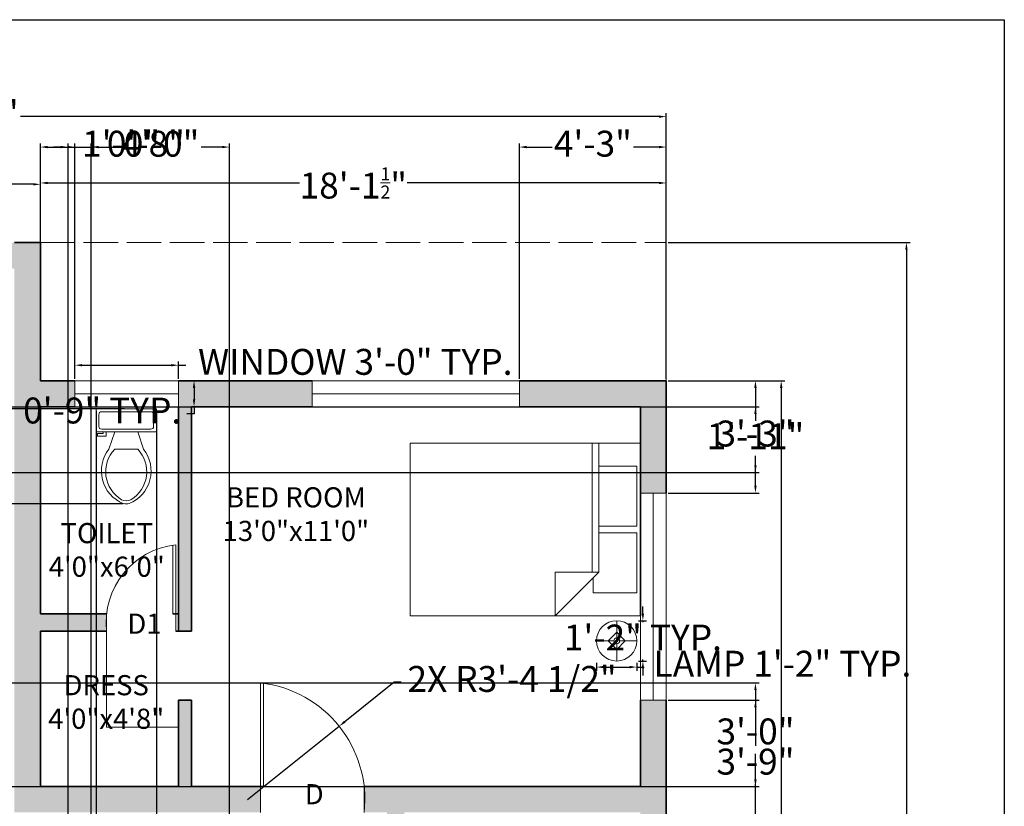
# Model space of a CAD drawing. Units: inches. Extents: x 1942 to 2601, y 2026 to 2623.
# Tile 5 of 5: x 2259 to 2601, y 2350 to 2623. Entities that reach past the tile are written whole.
import ezdxf

# ---------------------------------------------------------------- set-up
doc = ezdxf.new("R2010")
doc.units = ezdxf.units.IN
doc.linetypes.add('ACAD_ISO02W100', pattern=[15, 12, -3])
for name, color, linetype, lineweight in [('A-ANNO-DIMS', 2, 'Continuous', 18), ('A-ANNO-TEXT', 7, 'Continuous', 18), ('A-ANNO-TTLB', 7, 'Continuous', 25), ('A-AREA-IDEN', 7, 'Continuous', 25), ('A-DOOR', 4, 'Continuous', 18), ('A-FLOR-CASE', 8, 'Continuous', 18), ('A-FLOR-FIXT', 8, 'Continuous', 18), ('A-FLOR-OTLN', 8, 'ACAD_ISO02W100', 13), ('A-FURN', 8, 'Continuous', 18), ('A-GLAZ', 2, 'Continuous', 18), ('A-WALL', 7, 'Continuous', 35), ('A-WALL-PATT', 7, 'Continuous', 13)]:
    doc.layers.add(name, color=color, linetype=linetype, lineweight=lineweight)
doc.styles.get("Standard").update_dxf_attribs({"font": 'arial.ttf'})
doc.dimstyles.new('ISO-25', dxfattribs={"dimtxt": 9, "dimasz": 2.5, "dimexe": 1.25, "dimexo": 0.625, "dimgap": 2, "dimtad": 0, "dimtih": 1, "dimtoh": 1, "dimdec": 1, "dimlunit": 4, "dimtxsty": 'Standard', "dimcen": 2.5, "dimadec": 0, "dimazin": 0, "dimtfac": 0.5, "dimtdec": 1, "dimtmove": 0, "dimatfit": 3, "dimfxl": 1, "dimarcsym": 0})

# ---------------------------------------------------------------- blocks, each defined once
blk = doc.blocks.new('Bed - Queen')
for p, q in [((0, -80.00003), (0, 0)), ((0, 0), (59.99999, 0)), ((59.99999, 0), (59.99999, -80.00003)), ((7.99999, -1.2), (28.79998, -1.2)), ((7.99999, -14.4), (7.99999, -1.2)), ((28.79998, -1.2), (28.79998, -14.4)), ((31.19999, -1.2), (51.99999, -1.2)), ((31.19999, -14.4), (31.19999, -1.2)), ((51.99999, -1.2), (51.99999, -16.4)), ((0, -14.4), (44.8, -14.4)), ((44.8, -16.8), (0, -16.8)), ((59.99999, -29.6), (44.8, -14.4)), ((44.8, -14.4), (44.8, -29.6)), ((51.99999, -16.4), (46.79936, -16.4)), ((44.8, -29.6), (59.99999, -29.6)), ((59.99999, -80.00003), (0, -80.00003))]:
    blk.add_line(p, q)
blk = doc.blocks.new('Lamp - Table')
for p, q in [((0, 7), (0, 1)), ((-1, 0), (-7, 0)), ((0, 3), (-3, 0)), ((-3, 0), (0, -3)), ((3, 0), (0, 3)), ((0, -3), (3, 0)), ((1, 0), (7, 0)), ((0, -1), (0, -7))]:
    blk.add_line(p, q)
for radius in [7, 1]:
    blk.add_circle((0, 0), radius)
blk = doc.blocks.new('*U10')
for p, q in [((9.5, -6), (9.5, -2)), ((-10, -8.5), (-8, -8.5)), ((-10, -9.5), (-10, -8.5)), ((-7, -9.5), (-10, -9.5)), ((-8, -8.5), (-8, -8)), ((-7, -8), (-7, -9.5)), ((-4, -8), (-6, -14)), ((4, -8), (6, -14)), ((4, -14), (-4, -14))]:
    blk.add_line(p, q)
blk.add_lwpolyline([(10.5, -8), (10.5, 0), (-10.5, 0), (-10.5, -8)], close=True)
for points in [[(-9.5, -2), (-9.5, -6)], [(8.5, -1), (-8.5, -1)], [(-8.5, -7), (8.5, -7)]]:
    blk.add_lwpolyline(points)
for centre, radius, start, end in [((-8.62, -1.88), 0.884, 81.8699, 188.1301), ((8.62, -1.88), 0.884, 351.8699, 98.1301), ((-8.62, -6.12), 0.884, 171.8699, 278.1301), ((8.62, -6.12), 0.884, 261.8699, 8.1301), ((3.52, -21.58), 12.17, 141.4691, 247.9714), ((4.2, -21.82), 11.33, 136.3677, 238.9468), ((-3.52, -21.58), 12.17, 292.0284, 38.5307), ((-4.2, -21.82), 11.33, 301.053, 43.6321), ((0, -27.88), 4, 245.7318, 294.2682), ((0, -29), 4, 254.8605, 285.1395)]:
    blk.add_arc(centre, radius, start, end)
blk = doc.blocks.new('*D11')
at = {"layer": 'A-ANNO-DIMS', "color": 0, "lineweight": -2, "transparency": 16777216}
for p, q in [((2164.82, 2546.54), (2164.82, 2567.42)), ((2266.32, 2546.54), (2266.32, 2567.42)), ((2167.32, 2566.17), (2199.96, 2566.17)), ((2263.82, 2566.17), (2231.18, 2566.17))]:
    blk.add_line(p, q, dxfattribs=at)
at = {"layer": 'A-ANNO-DIMS', "color": 0, "transparency": 16777216}
for points in [[(2167.32, 2566.58), (2167.32, 2565.75), (2164.82, 2566.17)], [(2263.82, 2566.58), (2263.82, 2565.75), (2266.32, 2566.17)]]:
    blk.add_solid(points, dxfattribs=at)
at = {"layer": 'Defpoints', "color": 0, "transparency": 16777216}
for p in [(2266.32, 2566.17), (2164.82, 2545.91), (2266.32, 2545.91)]:
    blk.add_point(p, dxfattribs=at)
at = {"layer": 'A-ANNO-DIMS', "color": 0, "transparency": 16777216, "insert": (2215.57, 2566.17), "char_height": 9, "attachment_point": 5}
blk.add_mtext('8\'-5{\\H0.5x;\\S1/2;}"', dxfattribs=at)
blk = doc.blocks.new('*D13')
at = {"layer": 'A-ANNO-DIMS', "color": 0, "lineweight": -2, "transparency": 16777216}
for p, q in [((2266.32, 2498.54), (2266.32, 2567.89)), ((2268.82, 2566.64), (2356.39, 2566.64)), ((2481.32, 2566.64), (2393.75, 2566.64)), ((2483.82, 2498.54), (2483.82, 2567.89))]:
    blk.add_line(p, q, dxfattribs=at)
at = {"layer": 'A-ANNO-DIMS', "color": 0, "transparency": 16777216}
for points in [[(2268.82, 2567.06), (2268.82, 2566.23), (2266.32, 2566.64)], [(2481.32, 2567.06), (2481.32, 2566.23), (2483.82, 2566.64)]]:
    blk.add_solid(points, dxfattribs=at)
at = {"layer": 'Defpoints', "color": 0, "transparency": 16777216}
for p in [(2483.82, 2566.64), (2266.32, 2497.91), (2483.82, 2497.91)]:
    blk.add_point(p, dxfattribs=at)
at = {"layer": 'A-ANNO-DIMS', "color": 0, "transparency": 16777216, "insert": (2375.07, 2566.64), "char_height": 9, "attachment_point": 5}
blk.add_mtext('18\'-1{\\H0.5x;\\S1/2;}"', dxfattribs=at)
blk = doc.blocks.new('*D14')
at = {"layer": 'A-ANNO-DIMS', "color": 0, "lineweight": -2, "transparency": 16777216}
for p, q in [((1999.82, 2498.54), (1999.82, 2590.94)), ((2483.82, 2498.54), (2483.82, 2590.94)), ((2002.32, 2589.69), (2224.18, 2589.69)), ((2481.32, 2589.69), (2259.46, 2589.69))]:
    blk.add_line(p, q, dxfattribs=at)
at = {"layer": 'A-ANNO-DIMS', "color": 0, "transparency": 16777216}
for points in [[(2002.32, 2590.1), (2002.32, 2589.27), (1999.82, 2589.69)], [(2481.32, 2590.1), (2481.32, 2589.27), (2483.82, 2589.69)]]:
    blk.add_solid(points, dxfattribs=at)
at = {"layer": 'Defpoints', "color": 0, "transparency": 16777216}
for p in [(2483.82, 2589.69), (1999.82, 2497.91), (2483.82, 2497.91)]:
    blk.add_point(p, dxfattribs=at)
at = {"layer": 'A-ANNO-DIMS', "color": 0, "transparency": 16777216, "insert": (2241.82, 2589.69), "char_height": 9, "attachment_point": 5}
blk.add_mtext('40\'-4"', dxfattribs=at)
blk = doc.blocks.new('*D23')
at = {"layer": 'A-ANNO-DIMS', "color": 0, "lineweight": -2, "transparency": 16777216}
for p, q in [((2484.44, 2497.91), (2525.02, 2497.91)), ((2523.77, 2495.41), (2523.77, 2292.51)), ((2523.77, 2076.41), (2523.77, 2279.32)), ((2484.44, 2073.91), (2525.02, 2073.91))]:
    blk.add_line(p, q, dxfattribs=at)
at = {"layer": 'A-ANNO-DIMS', "color": 0, "transparency": 16777216}
for points in [[(2523.35, 2495.41), (2524.19, 2495.41), (2523.77, 2497.91)], [(2523.35, 2076.41), (2524.19, 2076.41), (2523.77, 2073.91)]]:
    blk.add_solid(points, dxfattribs=at)
at = {"layer": 'Defpoints', "color": 0, "transparency": 16777216}
for p in [(2483.82, 2497.91), (2483.82, 2073.91), (2523.77, 2073.91)]:
    blk.add_point(p, dxfattribs=at)
at = {"layer": 'A-ANNO-DIMS', "color": 0, "transparency": 16777216, "insert": (2523.77, 2285.91), "char_height": 9, "attachment_point": 5}
blk.add_mtext('35\'-4"', dxfattribs=at)
blk = doc.blocks.new('*D24')
at = {"layer": 'A-ANNO-DIMS', "color": 0, "lineweight": -2, "transparency": 16777216}
for p, q in [((2484.44, 2545.91), (2568.53, 2545.91)), ((2567.28, 2543.41), (2567.28, 2316.51)), ((2567.28, 2076.41), (2567.28, 2303.32)), ((2484.44, 2073.91), (2568.53, 2073.91))]:
    blk.add_line(p, q, dxfattribs=at)
at = {"layer": 'A-ANNO-DIMS', "color": 0, "transparency": 16777216}
for points in [[(2566.86, 2543.41), (2567.7, 2543.41), (2567.28, 2545.91)], [(2566.86, 2076.41), (2567.7, 2076.41), (2567.28, 2073.91)]]:
    blk.add_solid(points, dxfattribs=at)
at = {"layer": 'Defpoints', "color": 0, "transparency": 16777216}
for p in [(2483.82, 2545.91), (2483.82, 2073.91), (2567.28, 2073.91)]:
    blk.add_point(p, dxfattribs=at)
at = {"layer": 'A-ANNO-DIMS', "color": 0, "transparency": 16777216, "insert": (2567.28, 2309.91), "char_height": 9, "attachment_point": 5}
blk.add_mtext('39\'-4"', dxfattribs=at)
blk = doc.blocks.new('WIN-72IN')
for p, q in [((0, 0), (0, 9)), ((0, 9), (72, 9)), ((72, 0), (72, 9)), ((0, 4.5), (72, 4.5)), ((0, 0), (72, 0))]:
    blk.add_line(p, q)
blk = doc.blocks.new('DOOR-SINGLE-36IN')
for p, q in [((0, 9), (0, 45)), ((1, 9), (1, 44.88)), ((0, 0), (0, 9)), ((36, 0), (36, 9))]:
    blk.add_line(p, q)
blk.add_arc((-4.5, 4.5), 40.75, 353.6598, 83.6598)
blk = doc.blocks.new('DOOR-SINGLE-24IN')
for p, q in [((0, 6), (0, 30)), ((1, 6), (1, 29.87)), ((0, 6), (0, 0)), ((24, 6), (24, 0))]:
    blk.add_line(p, q)
blk.add_arc((-3, 3), 27.17, 353.6598, 83.6598)
blk = doc.blocks.new('WIN-36IN')
for p, q in [((0, 36), (9, 36)), ((0, 36), (0, 0)), ((4.5, 36), (4.5, 0)), ((9, 36), (9, 0)), ((0, 0), (9, 0))]:
    blk.add_line(p, q)
blk = doc.blocks.new('*D33')
at = {"layer": 'A-ANNO-DIMS', "color": 0, "lineweight": -2, "transparency": 16777216}
for p, q in [((2278.32, 2498.54), (2278.32, 2504.56)), ((2280.82, 2503.31), (2311.82, 2503.31)), ((2314.32, 2498.54), (2314.32, 2504.56)), ((2314.32, 2503.31), (2316.82, 2503.31))]:
    blk.add_line(p, q, dxfattribs=at)
at = {"layer": 'A-ANNO-DIMS', "color": 0, "transparency": 16777216}
for points in [[(2280.82, 2503.73), (2280.82, 2502.9), (2278.32, 2503.31)], [(2311.82, 2503.73), (2311.82, 2502.9), (2314.32, 2503.31)]]:
    blk.add_solid(points, dxfattribs=at)
at = {"layer": 'Defpoints', "color": 0, "transparency": 16777216}
for p in [(2314.32, 2503.31), (2278.32, 2497.91), (2314.32, 2497.91)]:
    blk.add_point(p, dxfattribs=at)
at = {"layer": 'A-ANNO-DIMS', "color": 0, "transparency": 16777216, "insert": (2375.76, 2503.31), "char_height": 9, "attachment_point": 5}
blk.add_mtext('WINDOW 3\'-0" TYP.', dxfattribs=at)
blk = doc.blocks.new('*D34')
at = {"layer": 'A-ANNO-DIMS', "color": 0, "lineweight": -2, "transparency": 16777216}
for p, q in [((2314.94, 2497.91), (2320.97, 2497.91)), ((2319.72, 2495.41), (2319.72, 2491.41)), ((2314.94, 2488.91), (2320.97, 2488.91)), ((2319.72, 2488.91), (2319.72, 2486.41)), ((2319.72, 2486.41), (2317.22, 2486.41))]:
    blk.add_line(p, q, dxfattribs=at)
at = {"layer": 'A-ANNO-DIMS', "color": 0, "transparency": 16777216}
for points in [[(2319.3, 2495.41), (2320.14, 2495.41), (2319.72, 2497.91)], [(2319.3, 2491.41), (2320.14, 2491.41), (2319.72, 2488.91)]]:
    blk.add_solid(points, dxfattribs=at)
at = {"layer": 'Defpoints', "color": 0, "transparency": 16777216}
for p in [(2314.32, 2497.91), (2314.32, 2488.91), (2319.72, 2488.91)]:
    blk.add_point(p, dxfattribs=at)
at = {"layer": 'A-ANNO-DIMS', "color": 0, "transparency": 16777216, "insert": (2287.79, 2486.41), "char_height": 9, "attachment_point": 5}
blk.add_mtext('0\'-9" TYP.', dxfattribs=at)
blk = doc.blocks.new('*D39')
at = {"layer": 'A-ANNO-DIMS', "color": 0, "lineweight": -2, "transparency": 16777216}
for p, q in [((2459.6, 2399.91), (2459.6, 2397.18)), ((2473.6, 2399.91), (2473.6, 2397.18)), ((2462.1, 2398.43), (2471.1, 2398.43)), ((2473.6, 2398.43), (2476.1, 2398.43))]:
    blk.add_line(p, q, dxfattribs=at)
at = {"layer": 'A-ANNO-DIMS', "color": 0, "transparency": 16777216}
for points in [[(2462.1, 2398.85), (2462.1, 2398.02), (2459.6, 2398.43)], [(2471.1, 2398.85), (2471.1, 2398.02), (2473.6, 2398.43)]]:
    blk.add_solid(points, dxfattribs=at)
at = {"layer": 'Defpoints', "color": 0, "transparency": 16777216}
for p in [(2459.6, 2400.53), (2473.6, 2400.53), (2473.6, 2398.43)]:
    blk.add_point(p, dxfattribs=at)
at = {"layer": 'A-ANNO-DIMS', "color": 0, "transparency": 16777216, "insert": (2524.2, 2398.43), "char_height": 9, "attachment_point": 5}
blk.add_mtext('LAMP 1\'-2" TYP.', dxfattribs=at)
blk = doc.blocks.new('*D40')
at = {"layer": 'A-ANNO-DIMS', "color": 0, "lineweight": -2, "transparency": 16777216}
for p, q in [((2475.7, 2417.03), (2475.7, 2419.53)), ((2474.23, 2414.53), (2476.95, 2414.53)), ((2475.7, 2414.53), (2475.7, 2414.06)), ((2474.23, 2400.53), (2476.95, 2400.53)), ((2475.7, 2400.53), (2475.7, 2401.01)), ((2475.7, 2398.03), (2475.7, 2395.53))]:
    blk.add_line(p, q, dxfattribs=at)
at = {"layer": 'A-ANNO-DIMS', "color": 0, "transparency": 16777216}
for points in [[(2475.28, 2417.03), (2476.12, 2417.03), (2475.7, 2414.53)], [(2475.28, 2398.03), (2476.12, 2398.03), (2475.7, 2400.53)]]:
    blk.add_solid(points, dxfattribs=at)
at = {"layer": 'Defpoints', "color": 0, "transparency": 16777216}
for p in [(2473.6, 2414.53), (2475.7, 2414.53), (2473.6, 2400.53)]:
    blk.add_point(p, dxfattribs=at)
at = {"layer": 'A-ANNO-DIMS', "color": 0, "transparency": 16777216, "insert": (2475.7, 2407.53), "char_height": 9, "attachment_point": 5}
blk.add_mtext('1\'-2" TYP.', dxfattribs=at)
blk = doc.blocks.new('*D58')
at = {"layer": 'A-ANNO-DIMS', "color": 0, "lineweight": -2, "transparency": 16777216}
for p, q in [((2266.32, 2498.54), (2266.32, 2580.37)), ((2278.32, 2498.54), (2278.32, 2580.37)), ((2268.82, 2579.12), (2275.82, 2579.12)), ((2278.32, 2579.12), (2280.82, 2579.12))]:
    blk.add_line(p, q, dxfattribs=at)
at = {"layer": 'A-ANNO-DIMS', "color": 0, "transparency": 16777216}
for points in [[(2268.82, 2579.54), (2268.82, 2578.7), (2266.32, 2579.12)], [(2275.82, 2579.54), (2275.82, 2578.7), (2278.32, 2579.12)]]:
    blk.add_solid(points, dxfattribs=at)
at = {"layer": 'Defpoints', "color": 0, "transparency": 16777216}
for p in [(2278.32, 2579.12), (2266.32, 2497.91), (2278.32, 2497.91)]:
    blk.add_point(p, dxfattribs=at)
at = {"layer": 'A-ANNO-DIMS', "color": 0, "transparency": 16777216, "insert": (2294.36, 2579.12), "char_height": 9, "attachment_point": 5}
blk.add_mtext('1\'-0"', dxfattribs=at)
blk = doc.blocks.new('*D59')
at = {"layer": 'A-ANNO-DIMS', "color": 0, "lineweight": -2, "transparency": 16777216}
for p, q in [((2432.82, 2498.54), (2432.82, 2580.37)), ((2483.82, 2498.54), (2483.82, 2580.37)), ((2435.32, 2579.12), (2444.18, 2579.12)), ((2481.32, 2579.12), (2472.46, 2579.12))]:
    blk.add_line(p, q, dxfattribs=at)
at = {"layer": 'A-ANNO-DIMS', "color": 0, "transparency": 16777216}
for points in [[(2435.32, 2579.54), (2435.32, 2578.7), (2432.82, 2579.12)], [(2481.32, 2579.54), (2481.32, 2578.7), (2483.82, 2579.12)]]:
    blk.add_solid(points, dxfattribs=at)
at = {"layer": 'Defpoints', "color": 0, "transparency": 16777216}
for p in [(2483.82, 2579.12), (2432.82, 2497.91), (2483.82, 2497.91)]:
    blk.add_point(p, dxfattribs=at)
at = {"layer": 'A-ANNO-DIMS', "color": 0, "transparency": 16777216, "insert": (2458.32, 2579.12), "char_height": 9, "attachment_point": 5}
blk.add_mtext('4\'-3"', dxfattribs=at)
blk = doc.blocks.new('*D60')
at = {"layer": 'A-ANNO-DIMS', "color": 0, "lineweight": -2, "transparency": 16777216}
for p, q in [((2484.44, 2497.91), (2516.07, 2497.91)), ((2514.82, 2495.41), (2514.82, 2485.01)), ((2514.82, 2461.41), (2514.82, 2471.82)), ((2484.44, 2458.91), (2516.07, 2458.91))]:
    blk.add_line(p, q, dxfattribs=at)
at = {"layer": 'A-ANNO-DIMS', "color": 0, "transparency": 16777216}
for points in [[(2514.4, 2495.41), (2515.24, 2495.41), (2514.82, 2497.91)], [(2514.4, 2461.41), (2515.24, 2461.41), (2514.82, 2458.91)]]:
    blk.add_solid(points, dxfattribs=at)
at = {"layer": 'Defpoints', "color": 0, "transparency": 16777216}
for p in [(2483.82, 2497.91), (2483.82, 2458.91), (2514.82, 2458.91)]:
    blk.add_point(p, dxfattribs=at)
at = {"layer": 'A-ANNO-DIMS', "color": 0, "transparency": 16777216, "insert": (2514.82, 2478.41), "char_height": 9, "attachment_point": 5}
blk.add_mtext('3\'-3"', dxfattribs=at)
blk = doc.blocks.new('*D61')
at = {"layer": 'A-ANNO-DIMS', "color": 0, "lineweight": -2, "transparency": 16777216}
for p, q in [((2484.44, 2386.91), (2516.07, 2386.91)), ((2514.82, 2384.41), (2514.82, 2371.01)), ((2514.82, 2344.41), (2514.82, 2357.82)), ((2484.44, 2341.91), (2516.07, 2341.91))]:
    blk.add_line(p, q, dxfattribs=at)
at = {"layer": 'A-ANNO-DIMS', "color": 0, "transparency": 16777216}
for points in [[(2514.4, 2384.41), (2515.24, 2384.41), (2514.82, 2386.91)], [(2514.4, 2344.41), (2515.24, 2344.41), (2514.82, 2341.91)]]:
    blk.add_solid(points, dxfattribs=at)
at = {"layer": 'Defpoints', "color": 0, "transparency": 16777216}
for p in [(2483.82, 2386.91), (2483.82, 2341.91), (2514.82, 2341.91)]:
    blk.add_point(p, dxfattribs=at)
at = {"layer": 'A-ANNO-DIMS', "color": 0, "transparency": 16777216, "insert": (2514.82, 2364.41), "char_height": 9, "attachment_point": 5}
blk.add_mtext('3\'-9"', dxfattribs=at)
blk = doc.blocks.new('*D67')
at = {"layer": 'A-ANNO-DIMS', "color": 0, "lineweight": -2, "transparency": 16777216}
for p, q in [((2275.92, 2167.54), (2275.92, 2580.37)), ((2284.02, 2167.54), (2284.02, 2580.37)), ((2273.42, 2579.12), (2270.92, 2579.12)), ((2275.92, 2579.12), (2284.02, 2579.12)), ((2286.52, 2579.12), (2289.02, 2579.12))]:
    blk.add_line(p, q, dxfattribs=at)
at = {"layer": 'A-ANNO-DIMS', "color": 0, "transparency": 16777216}
for points in [[(2273.42, 2579.54), (2273.42, 2578.7), (2275.92, 2579.12)], [(2286.52, 2579.54), (2286.52, 2578.7), (2284.02, 2579.12)]]:
    blk.add_solid(points, dxfattribs=at)
at = {"layer": 'Defpoints', "color": 0, "transparency": 16777216}
for p in [(2284.02, 2579.12), (2275.92, 2166.91), (2284.02, 2166.91)]:
    blk.add_point(p, dxfattribs=at)
at = {"layer": 'A-ANNO-DIMS', "color": 0, "transparency": 16777216, "insert": (2302.98, 2579.12), "char_height": 9, "attachment_point": 5}
blk.add_mtext('0\'-8"', dxfattribs=at)
blk = doc.blocks.new('*D68')
at = {"layer": 'A-ANNO-DIMS', "color": 0, "lineweight": -2, "transparency": 16777216}
for p, q in [((2284.02, 2167.54), (2284.02, 2580.37)), ((2332.02, 2167.54), (2332.02, 2580.37)), ((2286.52, 2579.12), (2293.88, 2579.12)), ((2329.52, 2579.12), (2322.16, 2579.12))]:
    blk.add_line(p, q, dxfattribs=at)
at = {"layer": 'A-ANNO-DIMS', "color": 0, "transparency": 16777216}
for points in [[(2286.52, 2579.54), (2286.52, 2578.7), (2284.02, 2579.12)], [(2329.52, 2579.54), (2329.52, 2578.7), (2332.02, 2579.12)]]:
    blk.add_solid(points, dxfattribs=at)
at = {"layer": 'Defpoints', "color": 0, "transparency": 16777216}
for p in [(2332.02, 2579.12), (2284.02, 2166.91), (2332.02, 2166.91)]:
    blk.add_point(p, dxfattribs=at)
at = {"layer": 'A-ANNO-DIMS', "color": 0, "transparency": 16777216, "insert": (2308.02, 2579.12), "char_height": 9, "attachment_point": 5}
blk.add_mtext('4\'-0"', dxfattribs=at)
blk = doc.blocks.new('*D72')
at = {"layer": 'A-ANNO-DIMS', "color": 0, "lineweight": -2, "transparency": 16777216}
for p, q in [((2174.44, 2392.91), (2516.07, 2392.91)), ((2514.82, 2390.41), (2514.82, 2381.51)), ((2514.82, 2359.41), (2514.82, 2368.32)), ((2174.44, 2356.91), (2516.07, 2356.91))]:
    blk.add_line(p, q, dxfattribs=at)
at = {"layer": 'A-ANNO-DIMS', "color": 0, "transparency": 16777216}
for points in [[(2514.4, 2390.41), (2515.24, 2390.41), (2514.82, 2392.91)], [(2514.4, 2359.41), (2515.24, 2359.41), (2514.82, 2356.91)]]:
    blk.add_solid(points, dxfattribs=at)
at = {"layer": 'Defpoints', "color": 0, "transparency": 16777216}
for p in [(2173.82, 2392.91), (2514.82, 2392.91), (2173.82, 2356.91)]:
    blk.add_point(p, dxfattribs=at)
at = {"layer": 'A-ANNO-DIMS', "color": 0, "transparency": 16777216, "insert": (2514.82, 2374.91), "char_height": 9, "attachment_point": 5}
blk.add_mtext('3\'-0"', dxfattribs=at)
blk = doc.blocks.new('*D74')
at = {"layer": 'A-ANNO-DIMS', "color": 0, "lineweight": -2, "transparency": 16777216}
for p, q in [((2009.44, 2488.91), (2516.07, 2488.91)), ((2514.82, 2486.41), (2514.82, 2484)), ((2514.82, 2468.55), (2514.82, 2470.96)), ((2029.44, 2466.05), (2516.07, 2466.05))]:
    blk.add_line(p, q, dxfattribs=at)
at = {"layer": 'A-ANNO-DIMS', "color": 0, "transparency": 16777216}
for points in [[(2514.4, 2486.41), (2515.24, 2486.41), (2514.82, 2488.91)], [(2514.4, 2468.55), (2515.24, 2468.55), (2514.82, 2466.05)]]:
    blk.add_solid(points, dxfattribs=at)
at = {"layer": 'Defpoints', "color": 0, "transparency": 16777216}
for p in [(2008.82, 2488.91), (2514.82, 2488.91), (2028.82, 2466.05)]:
    blk.add_point(p, dxfattribs=at)
at = {"layer": 'A-ANNO-DIMS', "color": 0, "transparency": 16777216, "insert": (2514.82, 2477.48), "char_height": 9, "attachment_point": 5}
blk.add_mtext('1\'-11"', dxfattribs=at)
blk = doc.blocks.new('*D75')
at = {"layer": 'A-ANNO-DIMS', "color": 0, "lineweight": -2, "transparency": 16777216}
for p, q in [((2285.65, 2487.5), (2285.65, 2041.66)), ((2306.65, 2487.5), (2306.65, 2041.66)), ((2288.15, 2042.91), (2304.15, 2042.91)), ((2306.65, 2042.91), (2309.15, 2042.91))]:
    blk.add_line(p, q, dxfattribs=at)
at = {"layer": 'A-ANNO-DIMS', "color": 0, "transparency": 16777216}
for points in [[(2288.15, 2043.33), (2288.15, 2042.5), (2285.65, 2042.91)], [(2304.15, 2043.33), (2304.15, 2042.5), (2306.65, 2042.91)]]:
    blk.add_solid(points, dxfattribs=at)
at = {"layer": 'Defpoints', "color": 0, "transparency": 16777216}
for p in [(2285.65, 2488.12), (2306.65, 2488.12), (2306.65, 2042.91)]:
    blk.add_point(p, dxfattribs=at)
at = {"layer": 'A-ANNO-DIMS', "color": 0, "transparency": 16777216, "insert": (2322.69, 2042.91), "char_height": 9, "attachment_point": 5}
blk.add_mtext('1\'-9"', dxfattribs=at)
blk = doc.blocks.new('*D76')
at = {"layer": 'A-ANNO-DIMS', "color": 0, "lineweight": -2, "transparency": 16777216}
for p, q in [((2295.53, 2488.12), (1967.57, 2488.12)), ((1968.82, 2485.62), (1968.82, 2478.23)), ((1968.82, 2457.66), (1968.82, 2465.04)), ((2295, 2455.16), (1967.57, 2455.16))]:
    blk.add_line(p, q, dxfattribs=at)
at = {"layer": 'A-ANNO-DIMS', "color": 0, "transparency": 16777216}
for points in [[(1968.4, 2485.62), (1969.24, 2485.62), (1968.82, 2488.12)], [(1968.4, 2457.66), (1969.24, 2457.66), (1968.82, 2455.16)]]:
    blk.add_solid(points, dxfattribs=at)
at = {"layer": 'Defpoints', "color": 0, "transparency": 16777216}
for p in [(1968.82, 2488.12), (2296.15, 2488.12), (2295.63, 2455.16)]:
    blk.add_point(p, dxfattribs=at)
at = {"layer": 'A-ANNO-DIMS', "color": 0, "transparency": 16777216, "insert": (1968.82, 2471.64), "char_height": 9, "attachment_point": 5}
blk.add_mtext('2\'-9"', dxfattribs=at)
blk = doc.blocks.new('*D78')
at = {"layer": 'A-ANNO-DIMS', "color": 0, "lineweight": -2, "transparency": 16777216}
for p, q in [((2389.23, 2393.14), (2372.09, 2379.43)), ((2391.73, 2393.14), (2389.23, 2393.14)), ((2338.32, 2352.41), (2370.14, 2377.87))]:
    blk.add_line(p, q, dxfattribs=at)
at = {"layer": 'A-ANNO-DIMS', "color": 0, "transparency": 16777216}
blk.add_solid([(2371.83, 2379.76), (2372.35, 2379.11), (2370.14, 2377.87)], dxfattribs=at)
at = {"layer": 'Defpoints', "color": 0, "transparency": 16777216}
for p in [(2370.14, 2377.87), (2338.32, 2352.41)]:
    blk.add_point(p, dxfattribs=at)
at = {"layer": 'A-ANNO-DIMS', "color": 0, "transparency": 16777216, "insert": (2430.23, 2393.14), "char_height": 9, "attachment_point": 5}
blk.add_mtext('2X R3\'-4 1/2"', dxfattribs=at)

msp = doc.modelspace()

# ---------------------------------------------------------------- hatches: boundary and pattern name
at = {"layer": 'A-WALL-PATT'}
h = msp.add_hatch(color=256, dxfattribs=at)
h.dxf.hatch_style = 1
h.paths.add_polyline_path([(2056.54, 2497.91), (1999.82, 2497.91), (1999.82, 2347.91), (2008.82, 2347.91), (2028.82, 2347.91), (2028.82, 2356.91), (2008.82, 2356.91), (2008.82, 2488.91), (2056.54, 2488.91)])
h.paths.add_polyline_path([(2173.82, 2356.91), (2164.82, 2356.91), (2076.82, 2356.91), (2076.82, 2347.91), (2096.82, 2347.91), (2105.82, 2347.91), (2164.82, 2347.91), (2173.82, 2347.91)])
h.paths.add_polyline_path([(2173.82, 2488.91), (2173.82, 2497.91), (2173.82, 2536.91), (2179.57, 2536.91), (2179.57, 2545.91), (2173.82, 2545.91), (2164.82, 2545.91), (2164.82, 2497.91), (2161.07, 2497.91), (2161.07, 2488.91), (2164.82, 2488.91), (2164.82, 2392.91), (2173.82, 2392.91)])
h.paths.add_polyline_path([(2125.07, 2497.91), (2116.54, 2497.91), (2116.54, 2488.91), (2125.07, 2488.91, -0.055385)])
h.paths.add_polyline_path([(2266.32, 2545.91), (2257.32, 2545.91), (2251.57, 2545.91), (2251.57, 2536.91), (2257.32, 2536.91), (2257.32, 2497.91), (2257.32, 2488.91), (2257.32, 2347.91), (2318.82, 2347.91), (2342.82, 2347.91), (2342.82, 2356.91), (2318.82, 2356.91), (2318.82, 2386.91), (2314.32, 2386.91), (2314.32, 2356.91), (2266.32, 2356.91), (2266.32, 2410.91), (2289.34, 2410.91, -0.055385), (2289.34, 2416.91), (2266.32, 2416.91), (2266.32, 2488.91), (2278.32, 2488.91), (2278.32, 2497.91), (2266.32, 2497.91)])
h.paths.add_polyline_path([(2360.82, 2497.91), (2314.32, 2497.91), (2314.32, 2488.91), (2314.32, 2416.91), (2314.32, 2410.91), (2318.82, 2410.91), (2318.82, 2488.91), (2360.82, 2488.91)])
h.paths.add_polyline_path([(2483.82, 2497.91), (2432.82, 2497.91), (2432.82, 2488.91), (2474.82, 2488.91), (2474.82, 2458.91), (2483.82, 2458.91)])
h.paths.add_polyline_path([(2483.82, 2386.91), (2474.82, 2386.91), (2474.82, 2356.91), (2378.82, 2356.91, -0.055385), (2378.82, 2347.91), (2386.82, 2347.91), (2386.82, 2299.91), (2386.82, 2293.91), (2394.45, 2293.91), (2394.45, 2299.91), (2392.82, 2299.91), (2392.82, 2347.91), (2474.82, 2347.91), (2474.82, 2341.91), (2483.82, 2341.91)])
h.paths.add_polyline_path([(2483.82, 2305.91), (2474.82, 2305.91), (2474.82, 2299.91), (2418.45, 2299.91, -0.055385), (2418.45, 2293.91), (2420.82, 2293.91), (2420.82, 2285.08, -0.055385), (2426.82, 2285.08), (2426.82, 2293.91), (2474.82, 2293.91), (2474.82, 2288.91), (2483.82, 2288.91)])

# ---------------------------------------------------------------- linework, layer by layer
at = {"layer": 'A-ANNO-TTLB'}
msp.add_lwpolyline([(1941.67, 2623.37), (2601.3, 2623.37), (2601.3, 2026.31), (1941.67, 2026.31)], close=True, dxfattribs=at)
at = {"layer": 'A-FLOR-CASE'}
for p, q in [((2289.34, 2410.91), (2289.34, 2377.58)), ((2289.34, 2377.58), (2314.32, 2377.58))]:
    msp.add_line(p, q, dxfattribs=at)
at = {"layer": 'A-FLOR-OTLN'}
for p in [(2266.32, 2545.91), (2483.82, 2497.91)]:
    msp.add_line(p, (2483.82, 2545.91), dxfattribs=at)
at = {"layer": 'A-WALL'}
for p, q in [((2257.32, 2545.91), (2266.32, 2545.91)), ((2266.32, 2497.91), (2266.32, 2545.91)), ((2266.32, 2497.91), (2278.32, 2497.91)), ((2314.32, 2497.91), (2360.82, 2497.91)), ((2432.82, 2497.91), (2483.82, 2497.91)), ((2483.82, 2497.91), (2483.82, 2458.91)), ((2266.32, 2488.91), (2266.32, 2416.91)), ((2266.32, 2488.91), (2278.32, 2488.91)), ((2314.32, 2488.91), (2314.32, 2416.91)), ((2318.82, 2488.91), (2318.82, 2410.91)), ((2318.82, 2488.91), (2360.82, 2488.91)), ((2432.82, 2488.91), (2474.82, 2488.91)), ((2474.82, 2488.91), (2474.82, 2416.22)), ((2266.32, 2416.91), (2289.34, 2416.91)), ((2312.34, 2416.91), (2314.32, 2416.91)), ((2314.32, 2416.91), (2314.32, 2410.91)), ((2266.32, 2410.91), (2289.34, 2410.91)), ((2266.32, 2410.91), (2266.32, 2356.91)), ((2313.34, 2410.91), (2314.32, 2410.91)), ((2314.32, 2410.91), (2318.82, 2410.91)), ((2314.32, 2386.91), (2314.32, 2356.91)), ((2314.32, 2386.91), (2318.82, 2386.91)), ((2318.82, 2386.91), (2318.82, 2356.91)), ((2474.82, 2386.91), (2474.82, 2356.91)), ((2483.82, 2386.91), (2483.82, 2341.91)), ((2314.32, 2356.91), (2266.32, 2356.91)), ((2318.82, 2356.91), (2343.82, 2356.91)), ((2378.82, 2356.91), (2474.82, 2356.91))]:
    msp.add_line(p, q, dxfattribs=at)

# ---------------------------------------------------------------- block references
at = {"layer": 'A-DOOR', "extrusion": (0, 0, -1), "zscale": -1}
msp.add_blockref('DOOR-SINGLE-24IN', (-2313.34, 2410.91), dxfattribs=at)
at = {"layer": 'A-DOOR'}
msp.add_blockref('DOOR-SINGLE-36IN', (2342.82, 2347.91), dxfattribs=at)
at = {"layer": 'A-FLOR-FIXT'}
msp.add_blockref('*U10', (2296.15, 2488.12), dxfattribs=at)
at = {"layer": 'A-FURN', "rotation": 270}
msp.add_blockref('Bed - Queen', (2474.82, 2476.22), dxfattribs=at)
at = {"layer": 'A-FURN'}
msp.add_blockref('Lamp - Table', (2466.6, 2407.53), dxfattribs=at)
at = {"layer": 'A-GLAZ'}
for name, p, rotation in [('WIN-36IN', (2278.32, 2497.91), 269.9999999999986), ('WIN-72IN', (2432.82, 2497.91), 180), ('WIN-72IN', (2474.82, 2458.91), 269.9999999999995)]:
    msp.add_blockref(name, p, dxfattribs=dict(at, rotation=rotation))

# ---------------------------------------------------------------- texts
at = {"layer": 'A-ANNO-TEXT', "char_height": 7, "attachment_point": 1}
for s, width, insert in [('\\pxqc;D1', 17.0257, (2293.97, 2417.01)), ('\\pxqc;D', 19.5389, (2351.7, 2357.76))]:
    msp.add_mtext_dynamic_manual_height_columns(s, width=width, gutter_width=12.5, heights=[0], dxfattribs=dict(at, insert=insert))
at = {"layer": 'A-AREA-IDEN', "char_height": 7, "attachment_point": 1}
for s, width, insert in [('\\pxqc;{\\fArial|b1|i0|c0|p34;BED ROOM\\P13\'0"x11\'0"}', 62.6624, (2323.78, 2460.91)), ('\\pxqc;{\\fArial|b1|i0|c0|p34;TOILET\\P4\'0"x6\'0"}', 37.7716, (2270.51, 2448.48)), ('\\pxqc;{\\fArial|b1|i0|c0|p34;DRESS\\P4\'0"x4\'8"}', 36.1751, (2271.11, 2395.64))]:
    msp.add_mtext_dynamic_manual_height_columns(s, width=width, gutter_width=12.5, heights=[0], dxfattribs=dict(at, insert=insert))

# ---------------------------------------------------------------- dimensions: what is measured, and where the dimension line sits
at = {"layer": 'A-ANNO-DIMS'}
for base, p1, p2, override, picture, middle in [((2483.82, 2589.69), (1999.82, 2497.91), (2483.82, 2497.91), {"dimclrd": 0, "dimclre": 0, "dimclrt": 0}, '*D14', (2241.82, 2589.69)), ((2278.32, 2579.12), (2266.32, 2497.91), (2278.32, 2497.91), {"dimdec": 1, "dimlfac": 1, "dimrnd": 0, "dimzin": 1, "dimdsep": 46, "dimlunit": 4, "dimfrac": 2}, '*D58', (2294.36, 2579.12)), ((2284.02, 2579.12), (2275.92, 2166.91), (2284.02, 2166.91), {"dimdec": 1, "dimlfac": 1, "dimrnd": 0, "dimzin": 1, "dimdsep": 46, "dimlunit": 4, "dimfrac": 2}, '*D67', (2302.98, 2579.12)), ((2332.02, 2579.12), (2284.02, 2166.91), (2332.02, 2166.91), {"dimdec": 1, "dimlfac": 1, "dimrnd": 0, "dimzin": 1, "dimdsep": 46, "dimlunit": 4, "dimfrac": 2}, '*D68', (2308.02, 2579.12)), ((2483.82, 2579.12), (2432.82, 2497.91), (2483.82, 2497.91), {"dimdec": 1, "dimlfac": 1, "dimrnd": 0, "dimzin": 1, "dimdsep": 46, "dimlunit": 4, "dimfrac": 2}, '*D59', (2458.32, 2579.12)), ((2266.32, 2566.17), (2164.82, 2545.91), (2266.32, 2545.91), {"dimclrd": 0, "dimclre": 0, "dimclrt": 0}, '*D11', (2215.57, 2566.17)), ((2483.82, 2566.64), (2266.32, 2497.91), (2483.82, 2497.91), {"dimclrd": 0, "dimclre": 0, "dimclrt": 0}, '*D13', (2375.07, 2566.64)), ((2306.65, 2042.91), (2285.65, 2488.12), (2306.65, 2488.12), {"dimdec": 1, "dimlfac": 1, "dimrnd": 0, "dimzin": 1, "dimdsep": 46, "dimlunit": 4, "dimfrac": 2}, '*D75', (2322.69, 2042.91))]:
    dim = msp.add_linear_dim(base=base, p1=p1, p2=p2, dimstyle='ISO-25', override=override, dxfattribs=at)
    dim.commit()
    dim.dimension.update_dxf_attribs({"geometry": picture, "text_midpoint": middle})
for base, p1, p2, override, picture, middle in [((2567.28, 2073.91), (2483.82, 2545.91), (2483.82, 2073.91), {"dimclrd": 0, "dimclre": 0, "dimclrt": 0}, '*D24', (2567.28, 2309.91)), ((2523.77, 2073.91), (2483.82, 2497.91), (2483.82, 2073.91), {"dimclrd": 0, "dimclre": 0, "dimclrt": 0}, '*D23', (2523.77, 2285.91)), ((2514.82, 2458.91), (2483.82, 2497.91), (2483.82, 2458.91), {"dimdec": 1, "dimlfac": 1, "dimrnd": 0, "dimzin": 1, "dimdsep": 46, "dimlunit": 4, "dimfrac": 2}, '*D60', (2514.82, 2478.41)), ((1968.82, 2488.12), (2295.63, 2455.16), (2296.15, 2488.12), {"dimdec": 1, "dimlfac": 1, "dimrnd": 0, "dimzin": 1, "dimdsep": 46, "dimlunit": 4, "dimfrac": 2}, '*D76', (1968.82, 2471.64)), ((2514.82, 2488.91), (2028.82, 2466.05), (2008.82, 2488.91), {"dimdec": 1, "dimlfac": 1, "dimrnd": 0, "dimzin": 1, "dimdsep": 46, "dimlunit": 4, "dimfrac": 2}, '*D74', (2514.82, 2477.48)), ((2514.82, 2392.91), (2173.82, 2356.91), (2173.82, 2392.91), {"dimdec": 1, "dimlfac": 1, "dimrnd": 0, "dimzin": 1, "dimdsep": 46, "dimlunit": 4, "dimfrac": 2}, '*D72', (2514.82, 2374.91)), ((2514.82, 2341.91), (2483.82, 2386.91), (2483.82, 2341.91), {"dimdec": 1, "dimlfac": 1, "dimrnd": 0, "dimzin": 1, "dimdsep": 46, "dimlunit": 4, "dimfrac": 2}, '*D61', (2514.82, 2364.41))]:
    dim = msp.add_linear_dim(base=base, p1=p1, p2=p2, angle=90, dimstyle='ISO-25', override=override, dxfattribs=at)
    dim.commit()
    dim.dimension.update_dxf_attribs({"geometry": picture, "text_midpoint": middle})
for base, p1, p2, text, picture, middle in [((2314.32, 2503.31), (2278.32, 2497.91), (2314.32, 2497.91), 'WINDOW <> TYP.', '*D33', (2375.76, 2503.31)), ((2473.6, 2398.43), (2459.6, 2400.53), (2473.6, 2400.53), 'LAMP <> TYP.', '*D39', (2524.2, 2398.43))]:
    dim = msp.add_linear_dim(base=base, p1=p1, p2=p2, text=text, dimstyle='ISO-25', override={"dimdec": 1, "dimlfac": 1, "dimrnd": 0, "dimzin": 1, "dimdsep": 46, "dimlunit": 4, "dimfrac": 2}, dxfattribs=at)
    dim.commit()
    dim.dimension.update_dxf_attribs({"geometry": picture, "text_midpoint": middle})
for base, p1, p2, angle, picture, middle in [((2319.72, 2488.91), (2314.32, 2497.91), (2314.32, 2488.91), 270, '*D34', (2287.79, 2486.41)), ((2475.7, 2414.53), (2473.6, 2400.53), (2473.6, 2414.53), 90, '*D40', (2475.7, 2407.53))]:
    dim = msp.add_linear_dim(base=base, p1=p1, p2=p2, angle=angle, text='<> TYP.', dimstyle='ISO-25', override={"dimdec": 1, "dimlfac": 1, "dimrnd": 0, "dimzin": 1, "dimdsep": 46, "dimlunit": 4, "dimfrac": 2}, dxfattribs=at)
    dim.commit()
    dim.dimension.update_dxf_attribs({"geometry": picture, "text_midpoint": middle})
dim = msp.add_radius_dim(center=(2338.3197, 2352.4145), mpoint=(2370.1399, 2377.8699), text='2X <>', dimstyle='ISO-25', override={"dimdec": 1, "dimlfac": 1, "dimrnd": 0, "dimzin": 1, "dimdsep": 46, "dimlunit": 4, "dimfrac": 2}, dxfattribs=at)
dim.commit()
dim.dimension.update_dxf_attribs({"geometry": '*D78', "text_midpoint": (2430.2323, 2393.1431), "dimtype": 164})

doc.saveas('drawing.dxf')
